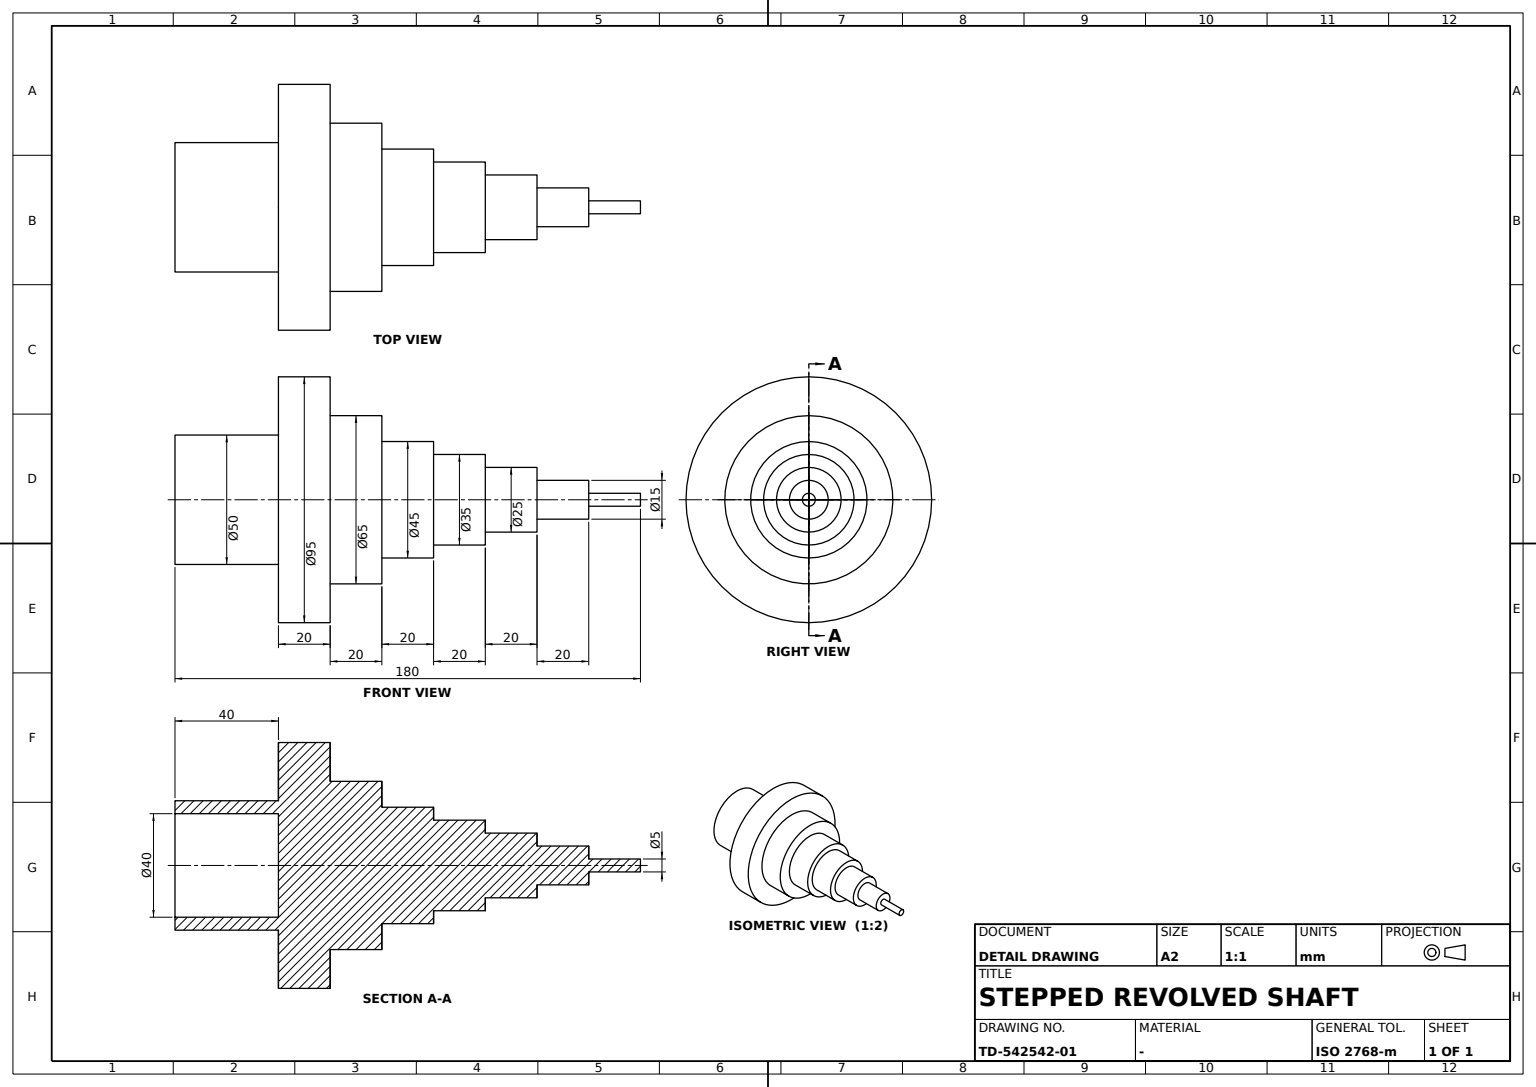
CATIA V5 part; units mm, degrees
sketch "Sketch1" plane through (0, 0, 0) normal (1, 0, 0) x (0, 1, 0)
  line L0 (0, 0) -> (0, 25)
  line L1 (0, 25) -> (40, 25)
  line L2 (40, 25) -> (40, 47.5)
  line L3 (40, 47.5) -> (60, 47.5)
  line L4 (60, 47.5) -> (60, 32.5)
  line L5 (60, 32.5) -> (80, 32.5)
  line L6 (80, 32.5) -> (80, 22.5)
  line L7 (80, 22.5) -> (100, 22.5)
  line L8 (100, 22.5) -> (100, 17.5)
  line L9 (100, 17.5) -> (120, 17.5)
  line L10 (120, 17.5) -> (120, 12.5)
  line L11 (120, 12.5) -> (140, 12.5)
  line L12 (140, 12.5) -> (140, 7.5)
  line L13 (140, 7.5) -> (160, 7.5)
  line L14 (160, 7.5) -> (160, 2.5)
  line L15 (160, 2.5) -> (180, 2.5)
  line L16 (180, 2.5) -> (180, 0)
  point P0 (180, 0)
  line L17 (180, 0) -> (0, 0)
  dimension "length L17" = 180
  dimension "length L0" = 25
  dimension "length L1" = 40
  dimension "length L3" = 20
  dimension "length L5" = 20
  dimension "length L7" = 20
  dimension "length L9" = 20
  dimension "length L11" = 20
  dimension "length L13" = 20
  dimension "length L16" = 2.5
  dimension "length L14" = 5
  dimension "length L12" = 5
  dimension "length L10" = 5
  dimension "length L8" = 5
  dimension "length L6" = 10
  dimension "length L4" = 15
  constraint vertical L0 y-axis
  constraint vertical L2 y-axis
  constraint vertical L4 y-axis
  constraint vertical L6 y-axis
  constraint vertical L8 y-axis
  constraint vertical L10 y-axis
  constraint vertical L12 y-axis
  constraint vertical L14 y-axis
  constraint vertical L16 y-axis
  constraint horizontal L1 x-axis
  constraint horizontal L3 x-axis
  constraint horizontal L5 x-axis
  constraint horizontal L7 x-axis
  constraint horizontal L9 x-axis
  constraint horizontal L11 x-axis
  constraint horizontal L13 x-axis
  constraint horizontal L15 x-axis
  constraint horizontal L17 x-axis
  constraint coincidence P0 x-axis
revolve "Shaft1" add sketch "Sketch1" angle 360 about L17
sketch "Sketch2" plane through (0, 0, 0) normal (0, -1, 0) x (1, 0, 0)
  point P0 (0, 0)
hole "Hole1" at (0, 0, 0) direction (0, 1, 0) diameter 40 depth 40
properties part number "design 2"
